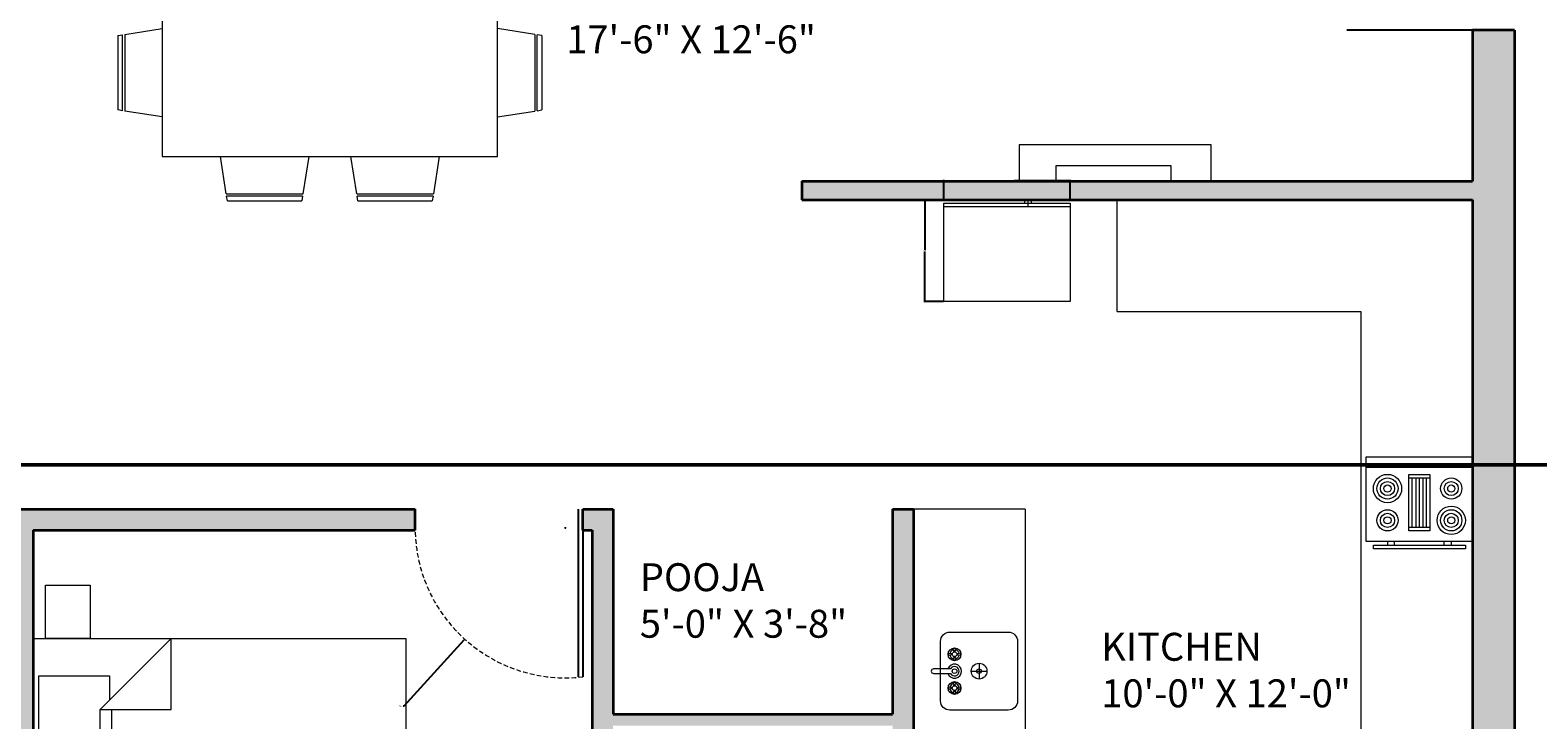
# Model space of a CAD drawing. Units: inches. Extents: x 1693 to 2974, y 2201 to 2965.
# Tile 10 of 24: x 1976 to 2299, y 2402 to 2550. Entities that reach past the tile are written whole.
import ezdxf

# ---------------------------------------------------------------- set-up
doc = ezdxf.new("R2010")
doc.units = ezdxf.units.IN
doc.header["$LTSCALE"] = 2
doc.header["$MEASUREMENT"] = 0
doc.linetypes.add('HIDDEN', pattern=[0.375, 0.25, -0.125])
for name, color, linetype, lineweight in [('A-ANNO-DIMS', 2, 'Continuous', 18), ('A-AREA-IDEN', 7, 'Continuous', 18), ('A-DOOR', 3, 'Continuous', 25), ('A-DOOR-SWNG', 3, 'HIDDEN', 13), ('A-EQPM', 8, 'Continuous', 18), ('A-FLOR-CASE', 32, 'Continuous', 18), ('A-FLOR-FIXT', 9, 'Continuous', 18), ('A-FURN', 8, 'Continuous', 18), ('A-WALL', 7, 'Continuous', 35)]:
    doc.layers.add(name, color=color, linetype=linetype, lineweight=lineweight)
doc.layers.add('A-WALL-PATT', color=251, linetype='Continuous', lineweight=13, true_color=0x636466)
doc.styles.get("Standard").update_dxf_attribs({"font": 'arial.ttf'})
doc.dimstyles.get("Standard").update_dxf_attribs({"dimtxt": 0.18, "dimasz": 0.18, "dimexe": 0.18, "dimexo": 0.0625, "dimgap": 0.09, "dimtad": 0, "dimtih": 1, "dimtoh": 1, "dimdec": 1, "dimzin": 0, "dimdsep": 46, "dimlunit": 3, "dimtxsty": 'Standard', "dimcen": 0.09, "dimadec": 0, "dimazin": 0, "dimtfac": 1, "dimtdec": 1, "dimtofl": 0, "dimtmove": 0, "dimatfit": 3, "dimfxl": 1, "dimtolj": 1, "dimtzin": 0, "dimarcsym": 0})

# ---------------------------------------------------------------- blocks, each defined once
blk = doc.blocks.new('Faucet - Bathroom top')
for p, q in [((-4.107, 0.125), (-4.375, 0.125)), ((-3.75, 0.4788), (-3.75, 0.75)), ((-3.5, 0.482), (-3.5, 0.75)), ((-3.1461, 0.125), (-2.875, 0.125)), ((3.143, 0.125), (2.875, 0.125)), ((3.5, 0.4788), (3.5, 0.75)), ((3.75, 0.482), (3.75, 0.75)), ((4.1039, 0.125), (4.375, 0.125)), ((-4.1039, -0.125), (-4.375, -0.125)), ((-3.75, -0.4821), (-3.75, -0.75)), ((-3.5, -0.4789), (-3.5, -0.75)), ((-3.143, -0.125), (-2.875, -0.125)), ((-0.5, -0.8639), (-0.5, -4.5)), ((0.5, -4.5), (0.5, -0.8631)), ((3.1461, -0.125), (2.875, -0.125)), ((3.5, -0.4821), (3.5, -0.75)), ((3.75, -0.4789), (3.75, -0.75)), ((4.107, -0.125), (4.375, -0.125))]:
    blk.add_line(p, q)
for centre, radius in [((-3.625, 0), 1.375), ((-4.625, 0), 0.2795), ((-3.625, 0), 0.5), ((-3.625, 1), 0.2795), ((-2.625, 0), 0.2795), ((0, 0), 0.5), ((3.625, 0), 1.375), ((2.625, 0), 0.2795), ((3.625, 0), 0.5), ((3.625, 1), 0.2795), ((4.625, 0), 0.2795), ((-3.625, -1), 0.2795), ((3.625, -1), 0.2795)]:
    blk.add_circle(centre, radius)
for centre, radius, start, end in [((-3.625, 0), 1, 105.2407, 164.2093), ((-3.625, 0), 1, 16.44125, 74.07887), ((0, 0), 1.5, 289.6514, 250.3603), ((0, 0), 1, 300.3431, 239.7554), ((3.625, 0), 1, 106.12, 164.0884), ((3.625, 0), 1, 16.23422, 73.90469), ((-3.625, 0), 1, 196.2342, 253.9047), ((-3.625, 0), 1, 286.12, 344.0884), ((3.625, 0), 1, 196.4413, 254.0789), ((3.625, 0), 1, 285.2407, 344.2093), ((0, -4.5), 0.5, 180, 0)]:
    blk.add_arc(centre, radius, start, end)
blk = doc.blocks.new('Range-Oven - 30 in top')
for p, q in [((0, -3), (30, -3)), ((12, -6), (18, -6)), ((13, -20), (13, -6)), ((14, -6), (14, -20)), ((15, -20), (15, -6)), ((16, -6), (16, -20)), ((17, -20), (17, -6)), ((18, -20), (12, -20)), ((6, -24), (6, -25)), ((8, -25), (8, -24)), ((22, -25), (22, -24)), ((24, -24), (24, -25))]:
    blk.add_line(p, q)
for points in [[(0, -24), (0, 0), (30, 0), (30, -24)], [(12, -21), (12, -5), (18, -5), (18, -21)], [(2, -26), (2, -25), (28, -25), (28, -26)]]:
    blk.add_lwpolyline(points, close=True)
for centre, radius in [((6, -9), 4), ((6, -9), 3), ((6, -9), 2), ((6, -9), 1), ((24, -9), 3), ((24, -9), 2), ((24, -9), 1), ((6, -18), 3), ((6, -18), 2), ((6, -18), 1), ((24, -18), 4), ((24, -18), 3), ((24, -18), 2), ((24, -18), 1)]:
    blk.add_circle(centre, radius)
blk = doc.blocks.new('Refrigerator-2 door - 36 in top')
for p, q in [((0, -26.999999), (36, -26.999999)), ((11, -27.999999), (11, -28.999999)), ((11, -28.999999), (13, -28.999999)), ((12, -26.999999), (12, -28.999999)), ((13, -28.999999), (13, -27.999999))]:
    blk.add_line(p, q)
blk.add_lwpolyline([(0, -27.999999), (0, 0), (36, 0), (36, -27.999999)], close=True)
blk = doc.blocks.new('Bed - Queen')
for p, q in [((0, -80.00003), (0, 0)), ((0, 0), (59.99999, 0)), ((59.99999, 0), (59.99999, -80.00003)), ((7.99999, -1.2), (28.79998, -1.2)), ((7.99999, -14.4), (7.99999, -1.2)), ((28.79998, -1.2), (28.79998, -14.4)), ((31.19999, -1.2), (51.99999, -1.2)), ((31.19999, -14.4), (31.19999, -1.2)), ((51.99999, -1.2), (51.99999, -16.4)), ((0, -14.4), (44.8, -14.4)), ((59.99999, -29.6), (44.8, -14.4)), ((44.8, -14.4), (44.8, -29.6)), ((44.8, -16.8), (0, -16.8)), ((51.99999, -16.4), (46.79936, -16.4)), ((44.8, -29.6), (59.99999, -29.6)), ((59.99999, -80.00003), (0, -80.00003))]:
    blk.add_line(p, q)
blk = doc.blocks.new('DINING-SET-72x36-6-SEAT')
for p, q in [((23.27, 53.5), (22.02, 45.5)), ((23.27, 53.5), (39.74, 53.5)), ((23.5, 55), (23.34, 54)), ((39.66, 54), (23.35, 54)), ((23.5, 55), (39.5, 55)), ((39.66, 54), (39.5, 55)), ((40.98, 45.5), (39.73, 53.5)), ((51.27, 53.5), (50.02, 45.5)), ((51.27, 53.5), (67.74, 53.5)), ((51.5, 55), (51.34, 54)), ((67.66, 54), (51.35, 54)), ((51.5, 55), (67.5, 55)), ((67.66, 54), (67.5, 55)), ((68.98, 45.5), (67.73, 53.5)), ((81.5, 45.5), (9.5, 45.5)), ((9.5, 45.5), (9.5, 9.5)), ((81.5, 9.5), (81.5, 45.5)), ((0, 35.5), (1, 35.66)), ((1, 19.34), (1, 35.65)), ((1.5, 35.73), (9.5, 36.98)), ((1.5, 35.73), (1.5, 19.26)), ((89.5, 35.73), (81.5, 36.98)), ((89.5, 35.73), (89.5, 19.26)), ((91, 35.5), (90, 35.66)), ((90, 19.34), (90, 35.65)), ((0, 35.5), (0, 19.5)), ((91, 35.5), (91, 19.5)), ((1, 19.34), (0, 19.5)), ((90, 19.34), (91, 19.5)), ((9.5, 18.02), (1.5, 19.27)), ((81.5, 18.02), (89.5, 19.27)), ((9.5, 9.5), (81.5, 9.5)), ((23.27, 1.5), (22.02, 9.5)), ((40.98, 9.5), (39.73, 1.5)), ((51.27, 1.5), (50.02, 9.5)), ((68.98, 9.5), (67.73, 1.5)), ((23.27, 1.5), (39.74, 1.5)), ((23.5, 0), (23.34, 1)), ((39.66, 1), (23.35, 1)), ((23.5, 0), (39.5, 0)), ((39.66, 1), (39.5, 0)), ((51.27, 1.5), (67.74, 1.5)), ((51.5, 0), (51.34, 1)), ((67.66, 1), (51.35, 1)), ((51.5, 0), (67.5, 0)), ((67.66, 1), (67.5, 0))]:
    blk.add_line(p, q)
blk = doc.blocks.new('NIGHTSTAND')
at = {"ltscale": 2}
blk.add_lwpolyline([(11.51, 0), (0, 0), (0, 9.62), (11.51, 9.62)], close=True, dxfattribs=at)
blk = doc.blocks.new('*D55')
at = {"layer": 'A-ANNO-DIMS', "color": 0, "lineweight": -2, "ltscale": 2, "transparency": 16777216}
for p, q in [((2171.72, 2513.91), (2171.72, 2518.1)), ((2171.9, 2517.92), (2183.74, 2517.92)), ((2198.69, 2517.92), (2186.85, 2517.92)), ((2198.87, 2513.91), (2198.87, 2518.1))]:
    blk.add_line(p, q, dxfattribs=at)
at = {"layer": 'A-ANNO-DIMS', "color": 0, "ltscale": 2, "transparency": 16777216}
for points in [[(2171.9, 2517.95), (2171.9, 2517.89), (2171.72, 2517.92)], [(2198.69, 2517.95), (2198.69, 2517.89), (2198.87, 2517.92)]]:
    blk.add_solid(points, dxfattribs=at)
at = {"layer": 'Defpoints', "color": 0, "ltscale": 2, "transparency": 16777216}
for p in [(2171.72, 2517.92), (2171.72, 2513.84), (2198.87, 2513.84)]:
    blk.add_point(p, dxfattribs=at)
at = {"layer": 'A-ANNO-DIMS', "color": 0, "ltscale": 2, "transparency": 16777216, "insert": (2185.3, 2517.92), "char_height": 0.18, "attachment_point": 5}
blk.add_mtext('\\A1;REFRIGERATOR 27 TYP.', dxfattribs=at)
blk = doc.blocks.new('*D56')
at = {"layer": 'A-ANNO-DIMS', "color": 0, "lineweight": -2, "ltscale": 2, "transparency": 16777216}
for p, q in [((2171.66, 2513.84), (2167.47, 2513.84)), ((2167.65, 2513.66), (2167.65, 2503.09)), ((2167.65, 2492.15), (2167.65, 2502.73)), ((2171.66, 2491.97), (2167.47, 2491.97))]:
    blk.add_line(p, q, dxfattribs=at)
at = {"layer": 'A-ANNO-DIMS', "color": 0, "ltscale": 2, "transparency": 16777216}
for points in [[(2167.62, 2513.66), (2167.68, 2513.66), (2167.65, 2513.84)], [(2167.62, 2492.15), (2167.68, 2492.15), (2167.65, 2491.97)]]:
    blk.add_solid(points, dxfattribs=at)
at = {"layer": 'Defpoints', "color": 0, "ltscale": 2, "transparency": 16777216}
for p in [(2171.72, 2513.84), (2167.65, 2491.97), (2171.72, 2491.97)]:
    blk.add_point(p, dxfattribs=at)
at = {"layer": 'A-ANNO-DIMS', "color": 0, "ltscale": 2, "transparency": 16777216, "insert": (2167.65, 2502.91), "char_height": 0.18, "attachment_point": 5}
blk.add_mtext('\\A1;22 TYP.', dxfattribs=at)
blk = doc.blocks.new('*D82')
at = {"layer": 'A-ANNO-DIMS', "color": 0, "lineweight": -2, "ltscale": 2, "transparency": 16777216}
for p, q in [((2615.67, 2906.08), (1693.46, 2906.08)), ((1693.64, 2905.9), (1693.64, 2582.94)), ((1693.64, 2259.62), (1693.64, 2582.58)), ((2096.17, 2259.44), (1693.46, 2259.44))]:
    blk.add_line(p, q, dxfattribs=at)
at = {"layer": 'A-ANNO-DIMS', "color": 0, "ltscale": 2, "transparency": 16777216}
for points in [[(1693.61, 2905.9), (1693.67, 2905.9), (1693.64, 2906.08)], [(1693.61, 2259.62), (1693.67, 2259.62), (1693.64, 2259.44)]]:
    blk.add_solid(points, dxfattribs=at)
at = {"layer": 'Defpoints', "color": 0, "ltscale": 2, "transparency": 16777216}
for p in [(1693.64, 2906.08), (2615.74, 2906.08), (2096.24, 2259.44)]:
    blk.add_point(p, dxfattribs=at)
at = {"layer": 'A-ANNO-DIMS', "color": 0, "ltscale": 2, "transparency": 16777216, "insert": (1693.64, 2582.76), "char_height": 0.18, "attachment_point": 5}
blk.add_mtext('\\A1;646.6', dxfattribs=at)
blk = doc.blocks.new('*D108')
at = {"layer": 'A-ANNO-DIMS', "color": 0, "lineweight": -2, "ltscale": 2, "transparency": 16777216}
for p, q in [((1752.74, 2457.09), (2973.12, 2457.09)), ((2972.94, 2457.27), (2972.94, 2457.45)), ((2972.94, 2457.45), (2973.12, 2457.45)), ((1752.74, 2456.73), (2973.12, 2456.73)), ((2972.94, 2456.55), (2972.94, 2456.37))]:
    blk.add_line(p, q, dxfattribs=at)
at = {"layer": 'A-ANNO-DIMS', "color": 0, "ltscale": 2, "transparency": 16777216}
for points in [[(2972.91, 2457.27), (2972.97, 2457.27), (2972.94, 2457.09)], [(2972.91, 2456.55), (2972.97, 2456.55), (2972.94, 2456.73)]]:
    blk.add_solid(points, dxfattribs=at)
at = {"layer": 'Defpoints', "color": 0, "ltscale": 2, "transparency": 16777216}
for p in [(1752.68, 2457.09), (2972.94, 2457.09), (1752.68, 2456.73)]:
    blk.add_point(p, dxfattribs=at)
at = {"layer": 'A-ANNO-DIMS', "color": 0, "ltscale": 2, "transparency": 16777216, "insert": (2973.44, 2457.45), "char_height": 0.18, "attachment_point": 5}
blk.add_mtext('\\A1;0.36', dxfattribs=at)
blk = doc.blocks.new('*D116')
at = {"layer": 'A-ANNO-DIMS', "color": 0, "lineweight": -2, "ltscale": 2, "transparency": 16777216}
for p, q in [((2090.39, 2443.38), (2090.57, 2443.38)), ((2090.48, 2443.29), (2090.48, 2443.47)), ((2055.87, 2405.11), (2068.73, 2419.32)), ((2055.69, 2405.11), (2055.87, 2405.11))]:
    blk.add_line(p, q, dxfattribs=at)
at = {"layer": 'A-ANNO-DIMS', "color": 0, "ltscale": 2, "transparency": 16777216}
blk.add_solid([(2068.71, 2419.34), (2068.75, 2419.3), (2068.85, 2419.46)], dxfattribs=at)
at = {"layer": 'Defpoints', "color": 0, "ltscale": 2, "transparency": 16777216}
for p in [(2090.48, 2443.38), (2068.85, 2419.46)]:
    blk.add_point(p, dxfattribs=at)
at = {"layer": 'A-ANNO-DIMS', "color": 0, "ltscale": 2, "transparency": 16777216, "insert": (2055.21, 2405.11), "char_height": 0.18, "attachment_point": 5}
blk.add_mtext('\\A1;R32.25', dxfattribs=at)

msp = doc.modelspace()

# ---------------------------------------------------------------- hatches: boundary and pattern name
at = {"layer": 'A-WALL-PATT', "ltscale": 2}
h = msp.add_hatch(color=256, dxfattribs=at)
h.dxf.hatch_style = 1
h.paths.add_polyline_path([(2294.2363, 2706.8449), (2248.9863, 2706.8449), (2248.9863, 2697.8449), (2285.2363, 2697.8449), (2285.2363, 2586.2648), (2294.2363, 2586.2648)])
h.paths.add_polyline_path([(2294.2363, 2550.2648), (2285.2363, 2550.2648), (2285.2363, 2517.8449), (2141.2363, 2517.8449), (2141.2363, 2513.8449), (2285.2363, 2513.8449), (2285.2363, 2369.8449), (2253.0704, 2369.8449), (2253.0704, 2366.8449), (2285.2363, 2366.8449), (2285.2363, 2298.8449), (2165.2363, 2298.8449), (2165.2363, 2366.8449), (2165.2363, 2369.8449), (2165.2363, 2447.3449), (2160.7363, 2447.3449), (2160.7363, 2403.3449), (2100.7363, 2403.3449), (2100.7363, 2447.3449), (2094.2363, 2447.3449), (2094.2363, 2442.8449), (2096.2363, 2442.8449), (2096.2363, 2362.1344), (2100.7363, 2362.1344), (2100.7363, 2400.8449), (2160.7363, 2400.8449), (2160.7363, 2298.8449), (2151.9207, 2298.8449), (2151.9207, 2289.8449), (2184.7363, 2289.8449), (2184.7363, 2276.6449), (2189.2363, 2276.6449), (2189.2363, 2289.8449), (2294.2363, 2289.8449)])
h.paths.add_polyline_path([(2048.023, 2298.8449), (1976.2363, 2298.8449), (1976.2363, 2442.8449), (2058.2363, 2442.8449, -0.00822734), (2058.2363, 2443.9061), (2058.2363, 2447.3449), (2004.7363, 2447.3449), (1969.7363, 2447.3449), (1969.7363, 2442.8449), (1971.7363, 2442.8449), (1971.7363, 2298.8449), (1966.0781, 2298.8449), (1966.0781, 2289.8449), (2048.023, 2289.8449)])
h.paths.add_polyline_path([(2127.9207, 2298.8449), (2100.7363, 2298.8449), (2100.7363, 2332.1344), (2096.2363, 2332.1344), (2096.2363, 2298.8449), (2084.023, 2298.8449), (2084.023, 2289.8449), (2096.2363, 2289.8449), (2096.2363, 2259.4449), (2114.3201, 2259.4449), (2114.3201, 2263.4449), (2100.7363, 2263.4449), (2100.7363, 2289.8449), (2127.9207, 2289.8449)])

# ---------------------------------------------------------------- linework, layer by layer
at = {"layer": 'A-DOOR', "ltscale": 2}
for p, q in [((2294.2363, 2550.2648), (2258.2363, 2550.2648)), ((2093.2363, 2447.3449), (2093.2363, 2411.3449)), ((2094.2363, 2447.3449), (2094.2363, 2411.3449))]:
    msp.add_line(p, q, dxfattribs=at)
at = {"layer": 'A-DOOR-SWNG', "ltscale": 2}
msp.add_arc((2090.4818, 2443.3755), 32.2499, 179.057238, 276.685387, dxfattribs=at)
at = {"layer": 'A-FLOR-CASE', "ltscale": 2}
for p, q in [((2208.9796, 2489.8449), (2208.9796, 2513.8449)), ((2189.2363, 2447.3449), (2165.2363, 2447.3449))]:
    msp.add_line(p, q, dxfattribs=at)
at = {"layer": 'A-FLOR-CASE'}
for p, q in [((2208.9796, 2489.8449), (2261.2363, 2489.8449)), ((2261.2363, 2489.8449), (2261.2363, 2369.8449)), ((2189.2363, 2447.3449), (2189.2363, 2369.8449))]:
    msp.add_line(p, q, dxfattribs=at)
at = {"layer": 'A-FLOR-FIXT', "ltscale": 2}
for p, q in [((2177.6129, 2412.568), (2181.0058, 2412.568)), ((2179.3093, 2414.2644), (2179.3093, 2410.8715))]:
    msp.add_line(p, q, dxfattribs=at)
msp.add_lwpolyline([(2173.0443, 2420.9585), (2185.5744, 2420.9585, -0.41421356), (2187.5744, 2418.9585), (2187.5744, 2406.1775, -0.41421356), (2185.5744, 2404.1775), (2173.0443, 2404.1775, -0.41421356), (2171.0443, 2406.1775), (2171.0443, 2418.9585, -0.41421356)], format="xyb", close=True, dxfattribs=at)
for radius in [1.6964, 0.4868]:
    msp.add_circle((2179.3093, 2412.568), radius, dxfattribs=at)
at = {"layer": 'A-FURN', "ltscale": 2}
for points in [[(2187.9445, 2517.8449), (2229.1257, 2517.8449), (2229.1257, 2525.6098), (2187.9445, 2525.6098)], [(2195.8163, 2517.8449), (2220.5181, 2517.8449), (2220.5181, 2521.0813), (2195.8163, 2521.0813)]]:
    msp.add_lwpolyline(points, close=True, dxfattribs=at)
at = {"layer": 'A-WALL', "ltscale": 2}
msp.add_line((2294.2363, 2550.2648), (2285.2363, 2550.2648), dxfattribs=at)
at = {"layer": 'A-WALL'}
for p, q in [((2285.2363, 2550.2648), (2285.2363, 2517.8449)), ((2294.2363, 2550.2648), (2294.2363, 2289.8449)), ((2141.2363, 2517.8449), (2285.2363, 2517.8449)), ((2141.2363, 2517.8449), (2141.2363, 2513.8449)), ((2141.2363, 2513.8449), (2285.2363, 2513.8449)), ((2285.2363, 2513.8449), (2285.2363, 2369.8449)), ((1969.7363, 2447.3449), (2058.2363, 2447.3449)), ((2004.7363, 2447.3449), (2058.2363, 2447.3449)), ((2058.2363, 2442.8449), (2058.2363, 2447.3449)), ((2094.2363, 2442.8449), (2094.2363, 2447.3449)), ((2094.2363, 2447.3449), (2096.2363, 2447.3449)), ((2094.2363, 2447.3449), (2100.7363, 2447.3449)), ((2100.7363, 2447.3449), (2100.7363, 2403.3449)), ((2160.7363, 2447.3449), (2165.2363, 2447.3449)), ((2160.7363, 2447.3449), (2160.7363, 2403.3449)), ((2160.7363, 2447.3449), (2165.2363, 2447.3449)), ((2165.2363, 2447.3449), (2165.2363, 2369.8449)), ((1976.2363, 2442.8449), (1976.2363, 2298.8449)), ((1976.2363, 2442.8449), (2058.2363, 2442.8449)), ((2094.2363, 2442.8449), (2096.2363, 2442.8449)), ((2096.2363, 2442.8449), (2096.2363, 2362.1344)), ((2100.7363, 2403.3449), (2160.7363, 2403.3449))]:
    msp.add_line(p, q, dxfattribs=at)

# ---------------------------------------------------------------- block references
at = {"layer": 'A-EQPM', "ltscale": 2, "xscale": 0.7541930673648309, "yscale": 0.7541930673648309, "zscale": 0.7541930673648309, "rotation": 180}
msp.add_blockref('Refrigerator-2 door - 36 in top', (2198.8714, 2491.9733), dxfattribs=at)
at = {"layer": 'A-EQPM', "ltscale": 2, "xscale": 0.7601168214309315, "yscale": 0.7601168214309315, "zscale": 0.7601168214309315}
msp.add_blockref('Range-Oven - 30 in top', (2262.4328, 2458.633), dxfattribs=at)
at = {"layer": 'A-FLOR-FIXT', "ltscale": 2, "rotation": 270}
msp.add_blockref('Faucet - Bathroom top', (2174.0422, 2412.5516), dxfattribs=at)
at = {"layer": 'A-FURN'}
msp.add_blockref('DINING-SET-72x36-6-SEAT', (1994.416, 2513.61), dxfattribs=at)
at = {"layer": 'A-FURN', "rotation": 270.0000000000031}
msp.add_blockref('NIGHTSTAND', (1978.8504, 2431.0522), dxfattribs=at)
at = {"layer": 'A-FURN', "ltscale": 2, "rotation": 89.99999999999999}
msp.add_blockref('Bed - Queen', (1976.2363, 2359.5424), dxfattribs=at)

# ---------------------------------------------------------------- texts
at = {"layer": 'A-AREA-IDEN', "ltscale": 2, "char_height": 6, "attachment_point": 1}
for s, insert in [('DINING\\P17\'-6" X 12\'-6"', (2090.6733, 2561.2974)), ('POOJA\\P5\'-0" X 3\'-8"', (2106.4678, 2435.743)), ('KITCHEN\\P10\'-0" X 12\'-0"', (2205.5356, 2420.7949))]:
    msp.add_mtext_dynamic_manual_height_columns(s, width=108.452746, gutter_width=1, heights=[0], dxfattribs=dict(at, insert=insert))

# ---------------------------------------------------------------- dimensions: what is measured, and where the dimension line sits
at = {"layer": 'A-ANNO-DIMS', "ltscale": 2}
for base, p1, p2, override, picture, middle in [((1693.6363, 2906.0761), (2096.2363, 2259.4449), (2615.7363, 2906.0761), {"dimdec": 1, "dimlfac": 1, "dimrnd": 0, "dimzin": 0, "dimdsep": 46, "dimlunit": 2}, '*D82', (1693.6363, 2582.7605)), ((2972.9363, 2457.0877), (1752.6754, 2456.7302), (1752.6754, 2457.0877), {"dimdec": 2, "dimlfac": 1, "dimrnd": 0, "dimzin": 0, "dimdsep": 46, "dimlunit": 2}, '*D108', (2973.44, 2457.4477))]:
    dim = msp.add_linear_dim(base=base, p1=p1, p2=p2, angle=90, dimstyle='Standard', override=override, dxfattribs=at)
    dim.commit()
    dim.dimension.update_dxf_attribs({"geometry": picture, "text_midpoint": middle})
for base, p1, p2, angle, text, picture, middle in [((2171.7204, 2517.9175), (2198.8714, 2513.8449), (2171.7204, 2513.8449), 180, 'REFRIGERATOR <> TYP.', '*D55', (2185.2959, 2517.9175)), ((2167.6478, 2491.9733), (2171.7204, 2513.8449), (2171.7204, 2491.9733), 270, '<> TYP.', '*D56', (2167.6478, 2502.9091))]:
    dim = msp.add_linear_dim(base=base, p1=p1, p2=p2, angle=angle, text=text, dimstyle='Standard', override={"dimdec": 0, "dimlfac": 1, "dimrnd": 0, "dimzin": 0, "dimdsep": 46, "dimlunit": 2}, dxfattribs=at)
    dim.commit()
    dim.dimension.update_dxf_attribs({"geometry": picture, "text_midpoint": middle})
dim = msp.add_radius_dim(center=(2090.4818, 2443.3755), mpoint=(2068.8487, 2419.4577), dimstyle='Standard', override={"dimdec": 2, "dimlfac": 1, "dimrnd": 0, "dimzin": 0, "dimdsep": 46, "dimlunit": 2}, dxfattribs=at)
dim.commit()
dim.dimension.update_dxf_attribs({"geometry": '*D116', "text_midpoint": (2055.2083, 2405.107), "dimtype": 164})

doc.saveas('drawing.dxf')
